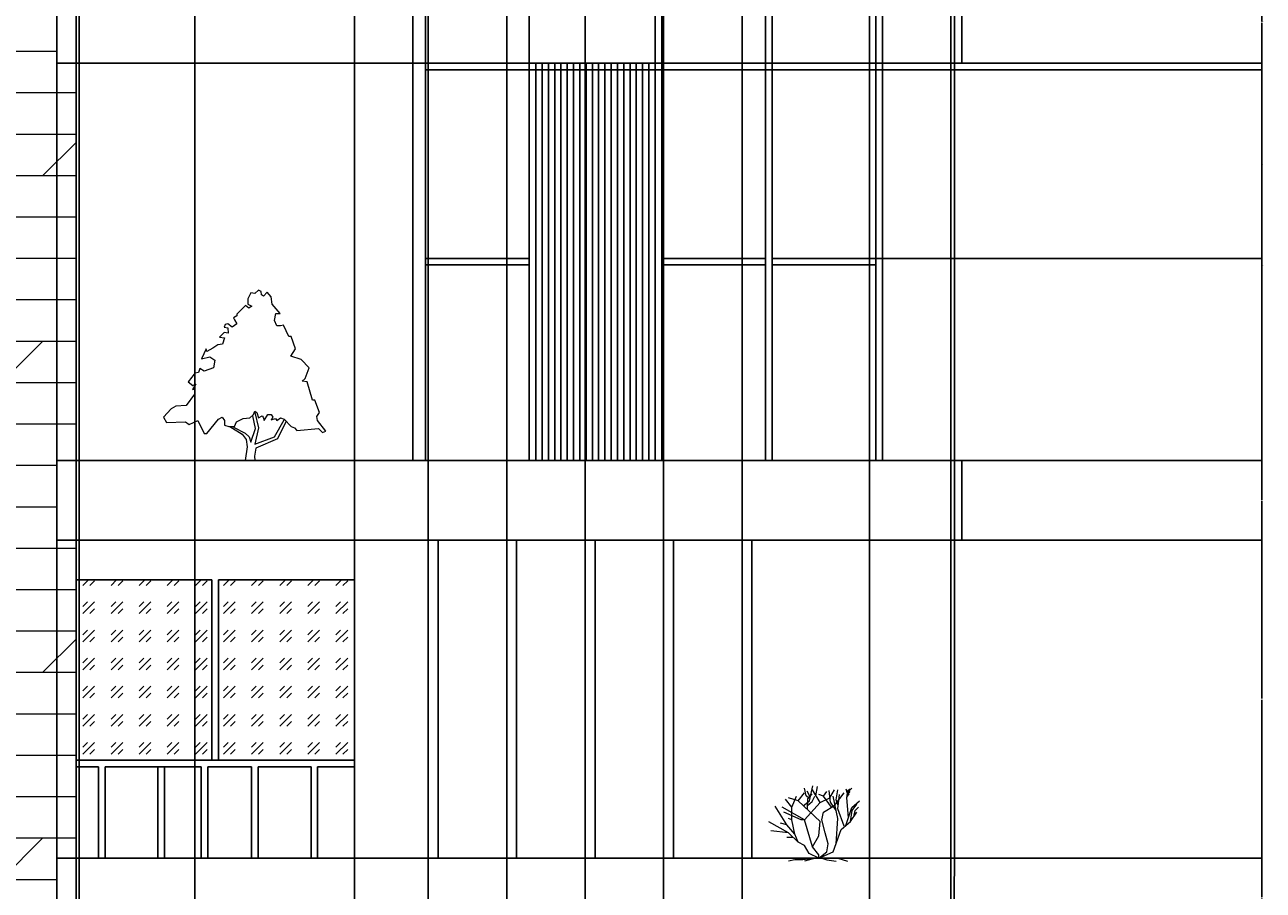
# Model space of a CAD drawing. Units: inches. Extents: x 250 to 1217, y -42 to 832.
# Tile 6 of 7: x 670 to 1043, y 309 to 571. Entities that reach past the tile are written whole.
import ezdxf

# ---------------------------------------------------------------- set-up
doc = ezdxf.new("R2010")
doc.units = ezdxf.units.IN
doc.header["$MEASUREMENT"] = 0
for name, color, linetype, lineweight in [('A-ANNO-DIMS', 2, 'Continuous', 18), ('A-ELEV', 7, 'Continuous', 25), ('A-ELEV-PATT', 8, 'Continuous', 13), ('L-PLNT', 3, 'Continuous', 13)]:
    doc.layers.add(name, color=color, linetype=linetype, lineweight=lineweight)
doc.styles.get("Standard").update_dxf_attribs({"font": 'arial.ttf'})
doc.dimstyles.get("Standard").update_dxf_attribs({"dimtxt": 0.18, "dimasz": 0.18, "dimexe": 0.18, "dimexo": 0.0625, "dimgap": 0.09, "dimtad": 0, "dimtih": 1, "dimtoh": 1, "dimdec": 4, "dimzin": 0, "dimdsep": 46, "dimtxsty": 'Standard', "dimcen": 0.09, "dimadec": 0, "dimazin": 0, "dimtfac": 1, "dimtdec": 4, "dimtofl": 0, "dimtmove": 0, "dimatfit": 3, "dimfxl": 1, "dimtolj": 1, "dimtzin": 0, "dimarcsym": 0})

# ---------------------------------------------------------------- blocks, each defined once
blk = doc.blocks.new('*U2')
for p, q in [((-11.433, 18.289), (-10.457, 22.749)), ((-9.48, 19.775), (-8.992, 22.592)), ((-16.8, 16.32), (-18.72, 18.72)), ((-14.88, 18.24), (-17.76, 19.2)), ((-16.8, 16.32), (-15.36, 19.68)), ((-14.88, 18.24), (-12.96, 20.64)), ((-12.471, 19.775), (-12.898, 22.044)), ((-11.677, 19.071), (-12.471, 19.775)), ((-11.28, 19.619), (-12.104, 21.184)), ((-12.043, 15.628), (-11.921, 18.836)), ((-11.921, 18.836), (-10.64, 20.401)), ((-10.579, 18.054), (-9.846, 19.697)), ((-8.16, 17.76), (-10.56, 21.6)), ((-7.2, 19.68), (-8.64, 20.16)), ((-8.16, 17.76), (-5.28, 19.2)), ((-7.2, 19.68), (-6.24, 21.12)), ((-4.8, 16.32), (-7.2, 19.68)), ((-5.086, 17.741), (-5.513, 21.34)), ((-5.28, 19.2), (-3.84, 21.6)), ((-2.88, 12.96), (-4.32, 19.68)), ((-3.84, 16.8), (-0.96, 20.64)), ((-3.377, 18.602), (-2.888, 21.575)), ((-2.88, 15.84), (-2.4, 20.16)), ((-0.508, 21.888), (-0.081, 20.558)), ((-0.203, 19.149), (0.102, 21.34)), ((0.346, 13.203), (-0.203, 19.149)), ((-0.142, 19.384), (0.59, 20.401)), ((-0.02, 20.01), (0.896, 21.105)), ((0.041, 20.714), (1.384, 22.044)), ((0.102, 21.34), (0.835, 21.888)), ((-18.24, 11.04), (-21.755, 16.655)), ((-12.96, 12.48), (-19.68, 16.32)), ((-16.8, 12.48), (-16.8, 16.32)), ((-8.16, 12), (-14.88, 18.24)), ((-13.325, 16.724), (-11.433, 18.289)), ((-12.96, 12.48), (-8.16, 17.76)), ((-11.982, 16.802), (-10.579, 18.054)), ((-7.2, 14.88), (-3.84, 16.8)), ((-3.377, 15.315), (-5.086, 17.819)), ((-2.766, 16.802), (-3.377, 18.602)), ((-0.96, 10.56), (-2.88, 15.84)), ((0.346, 13.203), (1.323, 16.254)), ((0.96, 12), (1.44, 15.36)), ((1.323, 16.254), (3.642, 18.289)), ((1.44, 15.36), (2.88, 17.28)), ((1.92, 13.44), (2.4, 15.36)), ((2.4, 15.36), (3.36, 16.32)), ((-17.76, 8.64), (-23.663, 11.961)), ((-18.24, 11.04), (-20.16, 11.52)), ((-13.92, 12.48), (-19.2, 14.88)), ((-16.8, 12.48), (-17.76, 12.96)), ((-15.84, 8.16), (-16.8, 12.48)), ((-12.96, 12.48), (-13.92, 12.48)), ((-10.56, 4.32), (-12.96, 12.48)), ((-8.64, 7.68), (-8.16, 12)), ((-7.68, 12.48), (-7.2, 14.88)), ((-6.72, 8.64), (-7.68, 12.48)), ((-3.36, 5.28), (-2.88, 12.96)), ((-1.92, 9.6), (0.96, 12)), ((-0.48, 10.8), (0.346, 13.203)), ((0.96, 12), (2.88, 14.88)), ((-17.76, 8.64), (-23.128, 9.222)), ((-15.84, 8.16), (-18.24, 11.04)), ((-14.88, 5.76), (-17.76, 8.64)), ((-14.88, 5.76), (-15.84, 8.16)), ((-10.56, 4.32), (-8.64, 7.68)), ((-5.76, 5.28), (-6.72, 8.64)), ((-4.32, 2.88), (-1.92, 9.6)), ((-16.32, 7.2), (-18.24, 7.2)), ((-12.96, 4.8), (-14.88, 5.76)), ((-11.52, 2.4), (-12.96, 4.8)), ((-8.64, 1.92), (-10.56, 4.32)), ((-6.24, 2.88), (-5.76, 5.28)), ((-15.84, 0.48), (-17.76, 0)), ((-13.44, 0.48), (-15.84, 0.48)), ((-9.6, 0.96), (-13.44, 0.48)), ((-9.6, 0.96), (-12.96, 0)), ((-8.64, 0.96), (-11.52, 2.4)), ((-9.6, 0.96), (-7.68, 0.96)), ((-8.64, 0.96), (-4.32, 2.88)), ((-8.64, 0.96), (-6.24, 2.88)), ((-8.64, 0.96), (-8.64, 1.92)), ((-8.64, 0.96), (-2.88, 0.96)), ((-7.68, 0.96), (-6.24, 0.48)), ((-6.24, 0.48), (-3.36, 0)), ((-2.88, 0.96), (0, 0))]:
    blk.add_line(p, q)
blk = doc.blocks.new('*U3')
for points in [[(22.0124, 137.721), (18.5475, 141.5624), (15.5282, 138.2446), (13.8028, 139.3505), (13.3714, 142.1153), (11.2148, 143.2214), (8.1954, 140.4564), (4.7447, 141.0094), (2.1567, 136.0326), (2.1567, 131.6088), (5.6074, 129.9499), (3.0193, 128.2909), (0.4313, 130.5029), (-6.9015, 123.3141), (-6.9015, 121.6552), (-9.9208, 119.9963), (-9.0581, 118.3373), (-6.9015, 115.0195), (-10.7835, 112.2546), (-14.6656, 115.0195), (-16.8222, 114.4665), (-17.6849, 112.2546), (-14.6656, 111.7016), (-14.2342, 107.2778), (-17.6065, 107.8307), (-21.5669, 103.9599), (-17.2536, 103.4069), (-18.9789, 97.8771), (-22.8609, 97.3241), (-27.1743, 94.5593), (-32.3504, 91.7944), (-32.7817, 94.0063), (-36.6638, 85.7116), (-29.7624, 87.3705), (-25.449, 84.6056), (-26.743, 77.9699), (-34.507, 75.205), (-37.9578, 77.4169), (-39.2518, 74.099), (-42.2711, 73.5461), (-44.8592, 70.2282), (-47.8786, 66.3574), (-43.9965, 63.0395), (-41.4085, 64.6985), (-44.3346, 59.8898), (-42.2089, 60.1377), (-42.5159, 55.7849), (-49.6039, 46.4502), (-58.2307, 45.8972), (-62.1127, 43.6853), (-68.5828, 36.4966), (-65.9947, 32.0727), (-50.0352, 32.6257), (-47.0159, 30.4138), (-39.6831, 33.7317), (-34.507, 22.6721), (-32.3504, 22.6721), (-22.4296, 34.8376), (-19.4102, 36.4966), (-17.2536, 33.7317), (-17.2536, 29.8608), (-13.8028, 28.7549), (-9.0581, 28.7549), (-7.3328, 32.6257), (-1.7254, 35.3906), (3.8821, 35.9436), (6.4701, 38.1555), (6.9014, 38.7085), (8.1954, 41.4734), (9.9208, 40.3674), (11.2148, 35.9436), (14.2341, 37.6025), (15.0968, 36.4966), (15.9595, 33.7317), (18.9789, 38.7085), (21.9982, 38.7085), (23.2922, 36.4966), (21.9982, 34.2847), (25.4489, 35.3906), (26.743, 33.7317), (29.7623, 35.9436), (32.7817, 34.8376), (38.8204, 28.7549), (41.4084, 27.6489), (43.5651, 25.437), (61.6813, 27.0959), (65.132, 23.7781), (67.7201, 24.884), (60.8186, 33.7317), (60.3873, 37.0495), (62.544, 40.3674), (58.662, 50.874), (56.5053, 50.874), (52.1919, 66.3574), (47.8785, 66.9103), (50.4665, 69.1222), (53.9172, 77.9699), (47.0158, 85.1586), (38.3891, 87.9235), (42.2711, 94.0063)], [(42.2711, 94.0063), (38.8204, 104.5129), (36.6637, 104.5129), (32.3503, 113.9135), (29.7623, 113.3605), (26.743, 113.3605), (24.5862, 117.7844), (25.8802, 123.8671), (29.331, 123.8671), (22.8609, 131.6088), (21.9982, 137.6916)], [(-9.9208, 28.2019), (0, 23.2251), (3.4507, 19.9072), (4.7447, 15.4834), (8.6267, 27.0959), (6.4701, 37.6025)], [(34.5071, 33.1787), (27.1743, 18.2483), (9.0581, 10.5066), (7.7641, 3.8708), (8.1954, 0)], [(8.1954, 40.3674), (11.2148, 27.6489), (8.1954, 13.8245), (24.5862, 19.9072), (32.7817, 34.2847)], [(-12.9401, 28.7549), (-2.588, 22.1191), (0.8626, 17.6953), (1.7253, 11.6125), (0, 0)]]:
    blk.add_lwpolyline(points)
blk = doc.blocks.new('*D15')
at = {"layer": 'A-ANNO-DIMS', "color": 0, "lineweight": -2, "transparency": 16777216}
for p, q in [((950.12, 318.93), (1043.08, 318.93)), ((1042.9, 318.75), (1042.9, 307.11)), ((1042.9, 295.11), (1042.9, 306.75)), ((926.12, 294.93), (1043.08, 294.93))]:
    blk.add_line(p, q, dxfattribs=at)
at = {"layer": 'A-ANNO-DIMS', "color": 0, "transparency": 16777216}
for points in [[(1042.87, 318.75), (1042.93, 318.75), (1042.9, 318.93)], [(1042.87, 295.11), (1042.93, 295.11), (1042.9, 294.93)]]:
    blk.add_solid(points, dxfattribs=at)
at = {"layer": 'Defpoints', "color": 0, "transparency": 16777216}
for p in [(950.06, 318.93), (1042.9, 318.93), (926.06, 294.93)]:
    blk.add_point(p, dxfattribs=at)
at = {"layer": 'A-ANNO-DIMS', "color": 0, "transparency": 16777216, "insert": (1042.9, 306.93), "char_height": 0.18, "attachment_point": 5}
blk.add_mtext('\\A1;24', dxfattribs=at)
blk = doc.blocks.new('*D16')
at = {"layer": 'A-ANNO-DIMS', "color": 0, "lineweight": -2, "transparency": 16777216}
for p, q in [((952.41, 414.93), (1043.08, 414.93)), ((1042.9, 414.75), (1042.9, 367.11)), ((1042.9, 319.11), (1042.9, 366.75)), ((950.12, 318.93), (1043.08, 318.93))]:
    blk.add_line(p, q, dxfattribs=at)
at = {"layer": 'A-ANNO-DIMS', "color": 0, "transparency": 16777216}
for points in [[(1042.87, 414.75), (1042.93, 414.75), (1042.9, 414.93)], [(1042.87, 319.11), (1042.93, 319.11), (1042.9, 318.93)]]:
    blk.add_solid(points, dxfattribs=at)
at = {"layer": 'Defpoints', "color": 0, "transparency": 16777216}
for p in [(952.34, 414.93), (1042.9, 414.93), (950.06, 318.93)]:
    blk.add_point(p, dxfattribs=at)
at = {"layer": 'A-ANNO-DIMS', "color": 0, "transparency": 16777216, "insert": (1042.9, 366.93), "char_height": 0.18, "attachment_point": 5}
blk.add_mtext('\\A1;96', dxfattribs=at)
blk = doc.blocks.new('*D17')
at = {"layer": 'A-ANNO-DIMS', "color": 0, "lineweight": -2, "transparency": 16777216}
for p, q in [((952.41, 438.93), (1043.08, 438.93)), ((1042.9, 438.75), (1042.9, 427.11)), ((1042.9, 415.11), (1042.9, 426.75)), ((952.41, 414.93), (1043.08, 414.93))]:
    blk.add_line(p, q, dxfattribs=at)
at = {"layer": 'A-ANNO-DIMS', "color": 0, "transparency": 16777216}
for points in [[(1042.87, 438.75), (1042.93, 438.75), (1042.9, 438.93)], [(1042.87, 415.11), (1042.93, 415.11), (1042.9, 414.93)]]:
    blk.add_solid(points, dxfattribs=at)
at = {"layer": 'Defpoints', "color": 0, "transparency": 16777216}
for p in [(952.34, 438.93), (1042.9, 438.93), (952.34, 414.93)]:
    blk.add_point(p, dxfattribs=at)
at = {"layer": 'A-ANNO-DIMS', "color": 0, "transparency": 16777216, "insert": (1042.9, 426.93), "char_height": 0.18, "attachment_point": 5}
blk.add_mtext('\\A1;24', dxfattribs=at)
blk = doc.blocks.new('*D18')
at = {"layer": 'A-ANNO-DIMS', "color": 0, "lineweight": -2, "transparency": 16777216}
for p, q in [((952.41, 558.93), (1043.08, 558.93)), ((1042.9, 558.75), (1042.9, 499.11)), ((1042.9, 439.11), (1042.9, 498.75)), ((952.41, 438.93), (1043.08, 438.93))]:
    blk.add_line(p, q, dxfattribs=at)
at = {"layer": 'A-ANNO-DIMS', "color": 0, "transparency": 16777216}
for points in [[(1042.87, 558.75), (1042.93, 558.75), (1042.9, 558.93)], [(1042.87, 439.11), (1042.93, 439.11), (1042.9, 438.93)]]:
    blk.add_solid(points, dxfattribs=at)
at = {"layer": 'Defpoints', "color": 0, "transparency": 16777216}
for p in [(952.34, 558.93), (1042.9, 558.93), (952.34, 438.93)]:
    blk.add_point(p, dxfattribs=at)
at = {"layer": 'A-ANNO-DIMS', "color": 0, "transparency": 16777216, "insert": (1042.9, 498.93), "char_height": 0.18, "attachment_point": 5}
blk.add_mtext('\\A1;120', dxfattribs=at)
blk = doc.blocks.new('*D19')
at = {"layer": 'A-ANNO-DIMS', "color": 0, "lineweight": -2, "transparency": 16777216}
for p, q in [((928.21, 583.67), (1043.08, 583.67)), ((1042.9, 583.49), (1042.9, 571.48)), ((1042.9, 559.11), (1042.9, 571.12)), ((952.41, 558.93), (1043.08, 558.93))]:
    blk.add_line(p, q, dxfattribs=at)
at = {"layer": 'A-ANNO-DIMS', "color": 0, "transparency": 16777216}
for points in [[(1042.87, 583.49), (1042.93, 583.49), (1042.9, 583.67)], [(1042.87, 559.11), (1042.93, 559.11), (1042.9, 558.93)]]:
    blk.add_solid(points, dxfattribs=at)
at = {"layer": 'Defpoints', "color": 0, "transparency": 16777216}
for p in [(928.15, 583.67), (1042.9, 583.67), (952.34, 558.93)]:
    blk.add_point(p, dxfattribs=at)
at = {"layer": 'A-ANNO-DIMS', "color": 0, "transparency": 16777216, "insert": (1042.9, 571.3), "char_height": 0.18, "attachment_point": 5}
blk.add_mtext('\\A1;24.747', dxfattribs=at)
blk = doc.blocks.new('*D27')
at = {"layer": 'A-ANNO-DIMS', "color": 0, "lineweight": -2, "transparency": 16777216}
for p, q in [((624.98, 174.99), (624.98, 831.77)), ((625.16, 831.59), (655.07, 831.59)), ((685.76, 831.59), (655.86, 831.59)), ((685.94, 176.49), (685.94, 831.77))]:
    blk.add_line(p, q, dxfattribs=at)
at = {"layer": 'A-ANNO-DIMS', "color": 0, "transparency": 16777216}
for points in [[(625.16, 831.62), (625.16, 831.56), (624.98, 831.59)], [(685.76, 831.62), (685.76, 831.56), (685.94, 831.59)]]:
    blk.add_solid(points, dxfattribs=at)
at = {"layer": 'Defpoints', "color": 0, "transparency": 16777216}
for p in [(685.94, 831.59), (685.94, 176.43), (624.98, 174.93)]:
    blk.add_point(p, dxfattribs=at)
at = {"layer": 'A-ANNO-DIMS', "color": 0, "transparency": 16777216, "insert": (655.46, 831.59), "char_height": 0.18, "attachment_point": 5}
blk.add_mtext('\\A1;60.96', dxfattribs=at)
blk = doc.blocks.new('*D28')
at = {"layer": 'A-ANNO-DIMS', "color": 0, "lineweight": -2, "transparency": 16777216}
for p, q in [((685.94, 176.49), (685.94, 831.77)), ((686.12, 831.59), (727.07, 831.59)), ((768.8, 831.59), (727.86, 831.59)), ((768.98, 162.99), (768.98, 831.77))]:
    blk.add_line(p, q, dxfattribs=at)
at = {"layer": 'A-ANNO-DIMS', "color": 0, "transparency": 16777216}
for points in [[(686.12, 831.62), (686.12, 831.56), (685.94, 831.59)], [(768.8, 831.62), (768.8, 831.56), (768.98, 831.59)]]:
    blk.add_solid(points, dxfattribs=at)
at = {"layer": 'Defpoints', "color": 0, "transparency": 16777216}
for p in [(768.98, 831.59), (685.94, 176.43), (768.98, 162.93)]:
    blk.add_point(p, dxfattribs=at)
at = {"layer": 'A-ANNO-DIMS', "color": 0, "transparency": 16777216, "insert": (727.46, 831.59), "char_height": 0.18, "attachment_point": 5}
blk.add_mtext('\\A1;83.04', dxfattribs=at)
blk = doc.blocks.new('*D29')
at = {"layer": 'A-ANNO-DIMS', "color": 0, "lineweight": -2, "transparency": 16777216}
for p, q in [((768.98, 162.99), (768.98, 831.77)), ((769.16, 831.59), (779.67, 831.59)), ((791.11, 831.59), (780.6, 831.59)), ((791.29, 174.99), (791.29, 831.77))]:
    blk.add_line(p, q, dxfattribs=at)
at = {"layer": 'A-ANNO-DIMS', "color": 0, "transparency": 16777216}
for points in [[(769.16, 831.62), (769.16, 831.56), (768.98, 831.59)], [(791.11, 831.62), (791.11, 831.56), (791.29, 831.59)]]:
    blk.add_solid(points, dxfattribs=at)
at = {"layer": 'Defpoints', "color": 0, "transparency": 16777216}
for p in [(791.29, 831.59), (791.29, 174.93), (768.98, 162.93)]:
    blk.add_point(p, dxfattribs=at)
at = {"layer": 'A-ANNO-DIMS', "color": 0, "transparency": 16777216, "insert": (780.13, 831.59), "char_height": 0.18, "attachment_point": 5}
blk.add_mtext('\\A1;22.303', dxfattribs=at)
blk = doc.blocks.new('*D30')
at = {"layer": 'A-ANNO-DIMS', "color": 0, "lineweight": -2, "transparency": 16777216}
for p, q in [((814.96, 174.99), (814.96, 831.77)), ((815.14, 831.59), (826.33, 831.59)), ((838.45, 831.59), (827.26, 831.59)), ((838.63, 174.99), (838.63, 831.77))]:
    blk.add_line(p, q, dxfattribs=at)
at = {"layer": 'A-ANNO-DIMS', "color": 0, "transparency": 16777216}
for points in [[(815.14, 831.62), (815.14, 831.56), (814.96, 831.59)], [(838.45, 831.62), (838.45, 831.56), (838.63, 831.59)]]:
    blk.add_solid(points, dxfattribs=at)
at = {"layer": 'Defpoints', "color": 0, "transparency": 16777216}
for p in [(838.63, 831.59), (814.96, 174.93), (838.63, 174.93)]:
    blk.add_point(p, dxfattribs=at)
at = {"layer": 'A-ANNO-DIMS', "color": 0, "transparency": 16777216, "insert": (826.8, 831.59), "char_height": 0.18, "attachment_point": 5}
blk.add_mtext('\\A1;23.674', dxfattribs=at)
blk = doc.blocks.new('*D31')
at = {"layer": 'A-ANNO-DIMS', "color": 0, "lineweight": -2, "transparency": 16777216}
for p, q in [((862.31, 174.99), (862.31, 831.77)), ((862.49, 831.59), (873.68, 831.59)), ((885.8, 831.59), (874.61, 831.59)), ((885.98, 174.99), (885.98, 831.77))]:
    blk.add_line(p, q, dxfattribs=at)
at = {"layer": 'A-ANNO-DIMS', "color": 0, "transparency": 16777216}
for points in [[(862.49, 831.62), (862.49, 831.56), (862.31, 831.59)], [(885.8, 831.62), (885.8, 831.56), (885.98, 831.59)]]:
    blk.add_solid(points, dxfattribs=at)
at = {"layer": 'Defpoints', "color": 0, "transparency": 16777216}
for p in [(885.98, 831.59), (862.31, 174.93), (885.98, 174.93)]:
    blk.add_point(p, dxfattribs=at)
at = {"layer": 'A-ANNO-DIMS', "color": 0, "transparency": 16777216, "insert": (874.15, 831.59), "char_height": 0.18, "attachment_point": 5}
blk.add_mtext('\\A1;23.674', dxfattribs=at)
blk = doc.blocks.new('*D32')
at = {"layer": 'A-ANNO-DIMS', "color": 0, "lineweight": -2, "transparency": 16777216}
for p, q in [((885.98, 174.99), (885.98, 831.77)), ((886.16, 831.59), (917.26, 831.59)), ((948.8, 831.59), (917.7, 831.59)), ((948.98, 174.99), (948.98, 831.77))]:
    blk.add_line(p, q, dxfattribs=at)
at = {"layer": 'A-ANNO-DIMS', "color": 0, "transparency": 16777216}
for points in [[(886.16, 831.62), (886.16, 831.56), (885.98, 831.59)], [(948.8, 831.62), (948.8, 831.56), (948.98, 831.59)]]:
    blk.add_solid(points, dxfattribs=at)
at = {"layer": 'Defpoints', "color": 0, "transparency": 16777216}
for p in [(948.98, 831.59), (885.98, 174.93), (948.98, 174.93)]:
    blk.add_point(p, dxfattribs=at)
at = {"layer": 'A-ANNO-DIMS', "color": 0, "transparency": 16777216, "insert": (917.48, 831.59), "char_height": 0.18, "attachment_point": 5}
blk.add_mtext('\\A1;63', dxfattribs=at)
blk = doc.blocks.new('*D33')
at = {"layer": 'A-ANNO-DIMS', "color": 0, "lineweight": -2, "transparency": 16777216}
for p, q in [((791.29, 414.99), (791.29, 831.77)), ((791.47, 831.59), (802.66, 831.59)), ((814.78, 831.59), (803.59, 831.59)), ((814.96, 414.99), (814.96, 831.77))]:
    blk.add_line(p, q, dxfattribs=at)
at = {"layer": 'A-ANNO-DIMS', "color": 0, "transparency": 16777216}
for points in [[(791.47, 831.62), (791.47, 831.56), (791.29, 831.59)], [(814.78, 831.62), (814.78, 831.56), (814.96, 831.59)]]:
    blk.add_solid(points, dxfattribs=at)
at = {"layer": 'Defpoints', "color": 0, "transparency": 16777216}
for p in [(814.96, 831.59), (791.29, 414.93), (814.96, 414.93)]:
    blk.add_point(p, dxfattribs=at)
at = {"layer": 'A-ANNO-DIMS', "color": 0, "transparency": 16777216, "insert": (803.12, 831.59), "char_height": 0.18, "attachment_point": 5}
blk.add_mtext('\\A1;23.674', dxfattribs=at)
blk = doc.blocks.new('*D34')
at = {"layer": 'A-ANNO-DIMS', "color": 0, "lineweight": -2, "transparency": 16777216}
for p, q in [((838.63, 414.99), (838.63, 831.77)), ((838.81, 831.59), (850.01, 831.59)), ((862.13, 831.59), (850.94, 831.59)), ((862.31, 414.99), (862.31, 831.77))]:
    blk.add_line(p, q, dxfattribs=at)
at = {"layer": 'A-ANNO-DIMS', "color": 0, "transparency": 16777216}
for points in [[(838.81, 831.62), (838.81, 831.56), (838.63, 831.59)], [(862.13, 831.62), (862.13, 831.56), (862.31, 831.59)]]:
    blk.add_solid(points, dxfattribs=at)
at = {"layer": 'Defpoints', "color": 0, "transparency": 16777216}
for p in [(862.31, 831.59), (838.63, 414.93), (862.31, 414.93)]:
    blk.add_point(p, dxfattribs=at)
at = {"layer": 'A-ANNO-DIMS', "color": 0, "transparency": 16777216, "insert": (850.47, 831.59), "char_height": 0.18, "attachment_point": 5}
blk.add_mtext('\\A1;23.674', dxfattribs=at)
blk = doc.blocks.new('*D37')
at = {"layer": 'A-ANNO-DIMS', "color": 0, "lineweight": -2, "transparency": 16777216}
for p, q in [((926.42, 499.99), (1043.08, 499.99)), ((1042.9, 499.81), (1042.9, 469.64)), ((1042.9, 439.11), (1042.9, 469.28)), ((928.42, 438.93), (1043.08, 438.93))]:
    blk.add_line(p, q, dxfattribs=at)
at = {"layer": 'A-ANNO-DIMS', "color": 0, "transparency": 16777216}
for points in [[(1042.87, 499.81), (1042.93, 499.81), (1042.9, 499.99)], [(1042.87, 439.11), (1042.93, 439.11), (1042.9, 438.93)]]:
    blk.add_solid(points, dxfattribs=at)
at = {"layer": 'Defpoints', "color": 0, "transparency": 16777216}
for p in [(926.36, 499.99), (1042.9, 499.99), (928.36, 438.93)]:
    blk.add_point(p, dxfattribs=at)
at = {"layer": 'A-ANNO-DIMS', "color": 0, "transparency": 16777216, "insert": (1042.9, 469.46), "char_height": 0.18, "attachment_point": 5}
blk.add_mtext('\\A1;61.06', dxfattribs=at)
blk = doc.blocks.new('*D50')
at = {"layer": 'A-ANNO-DIMS', "color": 0, "lineweight": -2, "transparency": 16777216}
for p, q in [((679.19, 318.99), (679.19, 831.77)), ((679.37, 831.59), (814.16, 831.59)), ((949.88, 831.59), (815.09, 831.59)), ((950.06, 318.99), (950.06, 831.77))]:
    blk.add_line(p, q, dxfattribs=at)
at = {"layer": 'A-ANNO-DIMS', "color": 0, "transparency": 16777216}
for points in [[(679.37, 831.62), (679.37, 831.56), (679.19, 831.59)], [(949.88, 831.62), (949.88, 831.56), (950.06, 831.59)]]:
    blk.add_solid(points, dxfattribs=at)
at = {"layer": 'Defpoints', "color": 0, "transparency": 16777216}
for p in [(950.06, 831.59), (679.19, 318.93), (950.06, 318.93)]:
    blk.add_point(p, dxfattribs=at)
at = {"layer": 'A-ANNO-DIMS', "color": 0, "transparency": 16777216, "insert": (814.62, 831.59), "char_height": 0.18, "attachment_point": 5}
blk.add_mtext('\\A1;270.87', dxfattribs=at)
blk = doc.blocks.new('*D52')
at = {"layer": 'A-ANNO-DIMS', "color": 0, "lineweight": -2, "transparency": 16777216}
for p, q in [((924.49, 199.65), (924.49, 831.77)), ((924.67, 831.59), (936.34, 831.59)), ((948.8, 831.59), (937.13, 831.59)), ((948.98, 198.99), (948.98, 831.77))]:
    blk.add_line(p, q, dxfattribs=at)
at = {"layer": 'A-ANNO-DIMS', "color": 0, "transparency": 16777216}
for points in [[(924.67, 831.62), (924.67, 831.56), (924.49, 831.59)], [(948.8, 831.62), (948.8, 831.56), (948.98, 831.59)]]:
    blk.add_solid(points, dxfattribs=at)
at = {"layer": 'Defpoints', "color": 0, "transparency": 16777216}
for p in [(948.98, 831.59), (924.49, 199.59), (948.98, 198.93)]:
    blk.add_point(p, dxfattribs=at)
at = {"layer": 'A-ANNO-DIMS', "color": 0, "transparency": 16777216, "insert": (936.74, 831.59), "char_height": 0.18, "attachment_point": 5}
blk.add_mtext('\\A1;24.49', dxfattribs=at)
blk = doc.blocks.new('*D55')
at = {"layer": 'A-ANNO-DIMS', "color": 0, "lineweight": -2, "transparency": 16777216}
for p, q in [((684.98, 438.99), (684.98, 831.77)), ((685.16, 831.59), (735.35, 831.59)), ((786.44, 831.59), (736.26, 831.59)), ((786.62, 438.99), (786.62, 831.77))]:
    blk.add_line(p, q, dxfattribs=at)
at = {"layer": 'A-ANNO-DIMS', "color": 0, "transparency": 16777216}
for points in [[(685.16, 831.62), (685.16, 831.56), (684.98, 831.59)], [(786.44, 831.62), (786.44, 831.56), (786.62, 831.59)]]:
    blk.add_solid(points, dxfattribs=at)
at = {"layer": 'Defpoints', "color": 0, "transparency": 16777216}
for p in [(786.62, 831.59), (684.98, 438.93), (786.62, 438.93)]:
    blk.add_point(p, dxfattribs=at)
at = {"layer": 'A-ANNO-DIMS', "color": 0, "transparency": 16777216, "insert": (735.8, 831.59), "char_height": 0.18, "attachment_point": 5}
blk.add_mtext('\\A1;101.64', dxfattribs=at)
blk = doc.blocks.new('*D56')
at = {"layer": 'A-ANNO-DIMS', "color": 0, "lineweight": -2, "transparency": 16777216}
for p, q in [((786.62, 438.99), (786.62, 831.77)), ((786.8, 831.59), (803.8, 831.59)), ((821.58, 831.59), (804.59, 831.59)), ((821.76, 438.99), (821.76, 831.77))]:
    blk.add_line(p, q, dxfattribs=at)
at = {"layer": 'A-ANNO-DIMS', "color": 0, "transparency": 16777216}
for points in [[(786.8, 831.62), (786.8, 831.56), (786.62, 831.59)], [(821.58, 831.62), (821.58, 831.56), (821.76, 831.59)]]:
    blk.add_solid(points, dxfattribs=at)
at = {"layer": 'Defpoints', "color": 0, "transparency": 16777216}
for p in [(821.76, 831.59), (786.62, 438.93), (821.76, 438.93)]:
    blk.add_point(p, dxfattribs=at)
at = {"layer": 'A-ANNO-DIMS', "color": 0, "transparency": 16777216, "insert": (804.19, 831.59), "char_height": 0.18, "attachment_point": 5}
blk.add_mtext('\\A1;35.14', dxfattribs=at)
blk = doc.blocks.new('*D57')
at = {"layer": 'A-ANNO-DIMS', "color": 0, "lineweight": -2, "transparency": 16777216}
for p, q in [((821.76, 438.99), (821.76, 831.77)), ((821.94, 831.59), (840.54, 831.59)), ((859.58, 831.59), (840.98, 831.59)), ((859.76, 438.99), (859.76, 831.77))]:
    blk.add_line(p, q, dxfattribs=at)
at = {"layer": 'A-ANNO-DIMS', "color": 0, "transparency": 16777216}
for points in [[(821.94, 831.62), (821.94, 831.56), (821.76, 831.59)], [(859.58, 831.62), (859.58, 831.56), (859.76, 831.59)]]:
    blk.add_solid(points, dxfattribs=at)
at = {"layer": 'Defpoints', "color": 0, "transparency": 16777216}
for p in [(859.76, 831.59), (821.76, 438.93), (859.76, 438.93)]:
    blk.add_point(p, dxfattribs=at)
at = {"layer": 'A-ANNO-DIMS', "color": 0, "transparency": 16777216, "insert": (840.76, 831.59), "char_height": 0.18, "attachment_point": 5}
blk.add_mtext('\\A1;38', dxfattribs=at)
blk = doc.blocks.new('*D58')
at = {"layer": 'A-ANNO-DIMS', "color": 0, "lineweight": -2, "transparency": 16777216}
for p, q in [((859.76, 438.99), (859.76, 831.77)), ((859.94, 831.59), (893.74, 831.59)), ((928.18, 831.59), (894.39, 831.59)), ((928.36, 438.99), (928.36, 831.77))]:
    blk.add_line(p, q, dxfattribs=at)
at = {"layer": 'A-ANNO-DIMS', "color": 0, "transparency": 16777216}
for points in [[(859.94, 831.62), (859.94, 831.56), (859.76, 831.59)], [(928.18, 831.62), (928.18, 831.56), (928.36, 831.59)]]:
    blk.add_solid(points, dxfattribs=at)
at = {"layer": 'Defpoints', "color": 0, "transparency": 16777216}
for p in [(928.36, 831.59), (859.76, 438.93), (928.36, 438.93)]:
    blk.add_point(p, dxfattribs=at)
at = {"layer": 'A-ANNO-DIMS', "color": 0, "transparency": 16777216, "insert": (894.06, 831.59), "char_height": 0.18, "attachment_point": 5}
blk.add_mtext('\\A1;68.6', dxfattribs=at)
blk = doc.blocks.new('*D87')
at = {"layer": 'A-ANNO-DIMS', "color": 0, "lineweight": -2, "transparency": 16777216}
for p, q in [((790.46, 438.99), (790.46, 831.77)), ((790.64, 831.59), (805.72, 831.59)), ((821.58, 831.59), (806.51, 831.59)), ((821.76, 438.99), (821.76, 831.77))]:
    blk.add_line(p, q, dxfattribs=at)
at = {"layer": 'A-ANNO-DIMS', "color": 0, "transparency": 16777216}
for points in [[(790.64, 831.62), (790.64, 831.56), (790.46, 831.59)], [(821.58, 831.62), (821.58, 831.56), (821.76, 831.59)]]:
    blk.add_solid(points, dxfattribs=at)
at = {"layer": 'Defpoints', "color": 0, "transparency": 16777216}
for p in [(821.76, 831.59), (790.46, 438.93), (821.76, 438.93)]:
    blk.add_point(p, dxfattribs=at)
at = {"layer": 'A-ANNO-DIMS', "color": 0, "transparency": 16777216, "insert": (806.11, 831.59), "char_height": 0.18, "attachment_point": 5}
blk.add_mtext('\\A1;31.30', dxfattribs=at)
blk = doc.blocks.new('*D88')
at = {"layer": 'A-ANNO-DIMS', "color": 0, "lineweight": -2, "transparency": 16777216}
for p, q in [((861.76, 438.99), (861.76, 831.77)), ((861.94, 831.59), (877.02, 831.59)), ((892.88, 831.59), (877.81, 831.59)), ((893.06, 438.99), (893.06, 831.77))]:
    blk.add_line(p, q, dxfattribs=at)
at = {"layer": 'A-ANNO-DIMS', "color": 0, "transparency": 16777216}
for points in [[(861.94, 831.62), (861.94, 831.56), (861.76, 831.59)], [(892.88, 831.62), (892.88, 831.56), (893.06, 831.59)]]:
    blk.add_solid(points, dxfattribs=at)
at = {"layer": 'Defpoints', "color": 0, "transparency": 16777216}
for p in [(893.06, 831.59), (861.76, 438.93), (893.06, 438.93)]:
    blk.add_point(p, dxfattribs=at)
at = {"layer": 'A-ANNO-DIMS', "color": 0, "transparency": 16777216, "insert": (877.41, 831.59), "char_height": 0.18, "attachment_point": 5}
blk.add_mtext('\\A1;31.30', dxfattribs=at)
blk = doc.blocks.new('*D89')
at = {"layer": 'A-ANNO-DIMS', "color": 0, "lineweight": -2, "transparency": 16777216}
for p, q in [((893.06, 438.99), (893.06, 831.77)), ((893.24, 831.59), (893.74, 831.59)), ((894.88, 831.59), (894.39, 831.59)), ((895.06, 438.99), (895.06, 831.77))]:
    blk.add_line(p, q, dxfattribs=at)
at = {"layer": 'A-ANNO-DIMS', "color": 0, "transparency": 16777216}
for points in [[(893.24, 831.62), (893.24, 831.56), (893.06, 831.59)], [(894.88, 831.62), (894.88, 831.56), (895.06, 831.59)]]:
    blk.add_solid(points, dxfattribs=at)
at = {"layer": 'Defpoints', "color": 0, "transparency": 16777216}
for p in [(895.06, 831.59), (893.06, 438.93), (895.06, 438.93)]:
    blk.add_point(p, dxfattribs=at)
at = {"layer": 'A-ANNO-DIMS', "color": 0, "transparency": 16777216, "insert": (894.06, 831.59), "char_height": 0.18, "attachment_point": 5}
blk.add_mtext('\\A1;2.00', dxfattribs=at)
blk = doc.blocks.new('*D90')
at = {"layer": 'A-ANNO-DIMS', "color": 0, "lineweight": -2, "transparency": 16777216}
for p, q in [((895.06, 438.99), (895.06, 831.77)), ((895.24, 831.59), (910.32, 831.59)), ((926.18, 831.59), (911.11, 831.59)), ((926.36, 438.99), (926.36, 831.77))]:
    blk.add_line(p, q, dxfattribs=at)
at = {"layer": 'A-ANNO-DIMS', "color": 0, "transparency": 16777216}
for points in [[(895.24, 831.62), (895.24, 831.56), (895.06, 831.59)], [(926.18, 831.62), (926.18, 831.56), (926.36, 831.59)]]:
    blk.add_solid(points, dxfattribs=at)
at = {"layer": 'Defpoints', "color": 0, "transparency": 16777216}
for p in [(926.36, 831.59), (895.06, 438.93), (926.36, 438.93)]:
    blk.add_point(p, dxfattribs=at)
at = {"layer": 'A-ANNO-DIMS', "color": 0, "transparency": 16777216, "insert": (910.71, 831.59), "char_height": 0.18, "attachment_point": 5}
blk.add_mtext('\\A1;31.30', dxfattribs=at)
blk = doc.blocks.new('*D91')
at = {"layer": 'A-ANNO-DIMS', "color": 0, "lineweight": -2, "transparency": 16777216}
for p, q in [((926.42, 556.93), (1043.08, 556.93)), ((1042.9, 556.75), (1042.9, 528.64)), ((1042.9, 500.17), (1042.9, 528.28)), ((926.42, 499.99), (1043.08, 499.99))]:
    blk.add_line(p, q, dxfattribs=at)
at = {"layer": 'A-ANNO-DIMS', "color": 0, "transparency": 16777216}
for points in [[(1042.87, 556.75), (1042.93, 556.75), (1042.9, 556.93)], [(1042.87, 500.17), (1042.93, 500.17), (1042.9, 499.99)]]:
    blk.add_solid(points, dxfattribs=at)
at = {"layer": 'Defpoints', "color": 0, "transparency": 16777216}
for p in [(926.36, 556.93), (1042.9, 556.93), (926.36, 499.99)]:
    blk.add_point(p, dxfattribs=at)
at = {"layer": 'A-ANNO-DIMS', "color": 0, "transparency": 16777216, "insert": (1042.9, 528.46), "char_height": 0.18, "attachment_point": 5}
blk.add_mtext('\\A1;56.94', dxfattribs=at)
blk = doc.blocks.new('*D92')
at = {"layer": 'A-ANNO-DIMS', "color": 0, "lineweight": -2, "transparency": 16777216}
for p, q in [((790.53, 556.93), (1043.08, 556.93)), ((1042.9, 556.75), (1042.9, 498.11)), ((1042.9, 439.11), (1042.9, 497.75)), ((790.53, 438.93), (1043.08, 438.93))]:
    blk.add_line(p, q, dxfattribs=at)
at = {"layer": 'A-ANNO-DIMS', "color": 0, "transparency": 16777216}
for points in [[(1042.87, 556.75), (1042.93, 556.75), (1042.9, 556.93)], [(1042.87, 439.11), (1042.93, 439.11), (1042.9, 438.93)]]:
    blk.add_solid(points, dxfattribs=at)
at = {"layer": 'Defpoints', "color": 0, "transparency": 16777216}
for p in [(790.46, 556.93), (1042.9, 556.93), (790.46, 438.93)]:
    blk.add_point(p, dxfattribs=at)
at = {"layer": 'A-ANNO-DIMS', "color": 0, "transparency": 16777216, "insert": (1042.9, 497.93), "char_height": 0.18, "attachment_point": 5}
blk.add_mtext('\\A1;118.00', dxfattribs=at)
blk = doc.blocks.new('*D98')
at = {"layer": 'A-ANNO-DIMS', "color": 0, "lineweight": -2, "transparency": 16777216}
for p, q in [((720.87, 583.82), (720.87, -41.6)), ((685.06, 582.86), (685.06, -41.6)), ((685.24, -41.42), (702.59, -41.42)), ((720.69, -41.42), (703.34, -41.42))]:
    blk.add_line(p, q, dxfattribs=at)
at = {"layer": 'A-ANNO-DIMS', "color": 0, "transparency": 16777216}
for points in [[(685.24, -41.39), (685.24, -41.45), (685.06, -41.42)], [(720.69, -41.39), (720.69, -41.45), (720.87, -41.42)]]:
    blk.add_solid(points, dxfattribs=at)
at = {"layer": 'Defpoints', "color": 0, "transparency": 16777216}
for p in [(720.87, 583.89), (685.06, 582.93), (720.87, -41.42)]:
    blk.add_point(p, dxfattribs=at)
at = {"layer": 'A-ANNO-DIMS', "color": 0, "transparency": 16777216, "insert": (702.97, -41.42), "char_height": 0.18, "attachment_point": 5}
blk.add_mtext('\\A1;35.81', dxfattribs=at)

msp = doc.modelspace()

# ---------------------------------------------------------------- hatches: boundary and pattern name
at = {"layer": 'A-ELEV-PATT'}
h = msp.add_hatch(dxfattribs=at)
h.set_pattern_fill('DOLMIT', color=256, scale=50)
h.paths.add_polyline_path([(684.9826, 558.9271), (679.1872, 558.9271), (679.1872, 582.9271), (685.0649, 582.9271), (685.0649, 678.9271), (679.1872, 678.9271), (679.1872, 702.9271), (630.7779, 702.9271), (630.7779, 678.9271), (625.0649, 678.9271), (625.0649, 582.9271), (630.7779, 582.9271), (630.7779, 558.9271), (624.9826, 558.9271), (624.9826, 438.9271), (630.7779, 438.9271), (630.7779, 414.9271), (624.9826, 414.9271), (624.9826, 318.9271), (630.7779, 318.9271), (630.7779, 294.9271), (624.9826, 294.9271), (624.9826, 198.9271), (630.7779, 198.9271), (630.7779, 174.9271), (624.9826, 174.9271), (624.9826, 78.9271), (684.9826, 78.9271), (684.9826, 174.9271), (679.1872, 174.9271), (679.1872, 198.9271), (683.6004, 198.9271), (684.9826, 198.9271), (684.9826, 294.9271), (679.1872, 294.9271), (679.1872, 318.9271), (684.9826, 318.9271), (684.9826, 414.9271), (679.1872, 414.9271), (679.1872, 438.9271), (684.9826, 438.9271)])
h = msp.add_hatch(dxfattribs=at)
h.set_pattern_fill('GOST_GLASS', color=256)
h.set_pattern_definition([(45, (144, 240), (8.48528, 0), [5, -7]), (45, (146.1213, 240), (8.48528, 0), [2, -10]), (45, (144, 242.1213), (8.48528, 0), [2, -10])])
h.paths.add_polyline_path([(725.9826, 402.9271), (684.9826, 402.9271), (684.9826, 348.4651), (722.7563, 348.4651), (725.9826, 348.4651)])
h.paths.add_polyline_path([(768.9826, 402.9271), (727.9826, 402.9271), (727.9826, 348.4651), (768.9826, 348.4651)])

# ---------------------------------------------------------------- linework, layer by layer
at = {"layer": 'A-ELEV'}
for p, q in [((679.1872, 582.9271), (679.1872, 558.9271)), ((952.3429, 558.9271), (952.3429, 582.9271)), ((679.1872, 558.9271), (952.3429, 558.9271)), ((684.9826, 558.9271), (684.9826, 438.9271)), ((786.6216, 438.9271), (786.6216, 558.9271)), ((790.4641, 499.991), (790.4641, 556.9271)), ((821.7635, 499.991), (821.7635, 556.9271)), ((823.7635, 558.9271), (823.7635, 438.9271)), ((825.6582, 558.9271), (825.6582, 438.9271)), ((827.5529, 558.9271), (827.5529, 438.9271)), ((829.4477, 558.9271), (829.4477, 438.9271)), ((831.3424, 558.9271), (831.3424, 438.9271)), ((833.2371, 558.9271), (833.2371, 438.9271)), ((835.1319, 558.9271), (835.1319, 438.9271)), ((837.0266, 558.9271), (837.0266, 438.9271)), ((838.9213, 558.9271), (838.9213, 438.9271)), ((840.8161, 558.9271), (840.8161, 438.9271)), ((842.7108, 558.9271), (842.7108, 438.9271)), ((844.6056, 558.9271), (844.6056, 438.9271)), ((846.5003, 558.9271), (846.5003, 438.9271)), ((848.395, 558.9271), (848.395, 438.9271)), ((850.2898, 558.9271), (850.2898, 438.9271)), ((852.1845, 558.9271), (852.1845, 438.9271)), ((854.0792, 558.9271), (854.0792, 438.9271)), ((855.974, 558.9271), (855.974, 438.9271)), ((857.8687, 558.9271), (857.8687, 438.9271)), ((859.7635, 558.9271), (859.7635, 438.9271)), ((859.7635, 558.9271), (859.7635, 438.9271)), ((859.7635, 558.9271), (859.7635, 438.9271)), ((859.7635, 558.9271), (859.7635, 438.9271)), ((861.7635, 499.991), (861.7635, 556.9271)), ((893.0628, 499.991), (893.0628, 556.9271)), ((895.0628, 499.991), (895.0628, 556.9271)), ((926.3621, 499.991), (926.3621, 556.9271)), ((928.3621, 438.9271), (928.3621, 558.9271)), ((790.4641, 499.991), (821.7635, 499.991)), ((790.4641, 438.9271), (790.4641, 497.991)), ((790.4641, 497.991), (821.7635, 497.991)), ((821.7635, 438.9271), (821.7635, 497.991)), ((861.7635, 499.991), (893.0628, 499.991)), ((861.7635, 438.9271), (861.7635, 497.991)), ((861.7635, 497.991), (893.0628, 497.991)), ((893.0628, 438.9271), (893.0628, 497.991)), ((895.0628, 499.991), (926.3621, 499.991)), ((895.0628, 438.9271), (895.0628, 497.991)), ((895.0628, 497.991), (926.3621, 497.991)), ((926.3621, 438.9271), (926.3621, 497.991)), ((679.1872, 438.9271), (679.1872, 414.9271)), ((679.1872, 438.9271), (952.3429, 438.9271)), ((952.3429, 438.9271), (952.3429, 414.9271)), ((679.1872, 414.9271), (952.3429, 414.9271)), ((679.1872, 414.9271), (888.9826, 414.9271)), ((684.9826, 414.9271), (684.9826, 318.9271)), ((791.2851, 414.9271), (791.2851, 318.9271)), ((794.2851, 414.9271), (794.2851, 318.9271)), ((814.9595, 414.9271), (814.9595, 318.9271)), ((817.9595, 414.9271), (817.9595, 318.9271)), ((838.6339, 414.9271), (838.6339, 318.9271)), ((841.6339, 414.9271), (841.6339, 318.9271)), ((862.3082, 414.9271), (862.3082, 318.9271)), ((865.3082, 414.9271), (865.3082, 318.9271)), ((885.9826, 414.9271), (885.9826, 318.9271)), ((888.9826, 414.9271), (888.9826, 318.9271)), ((725.9826, 402.9271), (684.9826, 402.9271)), ((725.9826, 402.9271), (725.9826, 348.4651)), ((727.9826, 402.9271), (727.9826, 348.4651)), ((727.9826, 402.9271), (768.9826, 402.9271)), ((768.9826, 402.9271), (727.9826, 402.9271)), ((768.9826, 402.9271), (768.9826, 318.9271)), ((722.7563, 348.4651), (684.9826, 348.4651)), ((768.9826, 348.4651), (708.9826, 348.4651)), ((691.7563, 346.4651), (684.9826, 346.4651)), ((691.7563, 346.4651), (691.7563, 318.9271)), ((693.7563, 346.4651), (693.7563, 318.9271)), ((709.684, 346.4651), (693.7563, 346.4651)), ((722.7563, 346.4651), (708.9826, 346.4651)), ((709.684, 346.4651), (709.684, 318.9271)), ((722.7563, 346.4651), (711.684, 346.4651)), ((711.684, 346.4651), (711.684, 318.9271)), ((722.7563, 346.4651), (722.7563, 318.9271)), ((737.9826, 346.4651), (724.7563, 346.4651)), ((724.7563, 346.4651), (724.7563, 318.9271)), ((737.9826, 346.4651), (737.9826, 318.9271)), ((739.9826, 346.4651), (739.9826, 318.9271)), ((755.9103, 346.4651), (739.9826, 346.4651)), ((755.9103, 346.4651), (755.9103, 318.9271)), ((768.9826, 346.4651), (757.9103, 346.4651)), ((757.9103, 346.4651), (757.9103, 318.9271)), ((679.1872, 318.9271), (679.1872, 294.9271)), ((679.1872, 318.9271), (948.9826, 318.9271))]:
    msp.add_line(p, q, dxfattribs=at)
msp.add_lwpolyline([(948.9826, 198.9271), (950.0561, 318.9271), (679.1872, 318.9271)], dxfattribs=at)

# ---------------------------------------------------------------- block references
at = {"layer": 'L-PLNT', "xscale": 0.3589292991008459, "yscale": 0.3589292991008459, "zscale": 0.3589292991008459}
msp.add_blockref('*U3', (736.0246, 438.9271), dxfattribs=at)
at = {"layer": 'L-PLNT'}
msp.add_blockref('*U2', (917.7694, 317.9671), dxfattribs=at)

# ---------------------------------------------------------------- dimensions: what is measured, and where the dimension line sits
at = {"layer": 'A-ANNO-DIMS'}
for base, p1, p2, override, picture, middle in [((685.944, 831.5941), (624.9826, 174.9271), (685.944, 176.4321), {"dimdec": 2, "dimlfac": 1, "dimrnd": 0, "dimzin": 0, "dimdsep": 46, "dimlunit": 2}, '*D27', (655.4633, 831.5941)), ((950.0561, 831.5941), (679.1872, 318.9271), (950.0561, 318.9271), {"dimdec": 2, "dimlfac": 1, "dimrnd": 0, "dimzin": 0, "dimdsep": 46, "dimlunit": 2}, '*D50', (814.6217, 831.5941)), ((786.6216, 831.5941), (684.9826, 438.9271), (786.6216, 438.9271), {"dimdec": 2, "dimlfac": 1, "dimrnd": 0, "dimzin": 0, "dimdsep": 46, "dimlunit": 2}, '*D55', (735.8021, 831.5941)), ((768.9826, 831.5941), (685.944, 176.4321), (768.9826, 162.9271), {"dimdec": 2, "dimlfac": 1, "dimrnd": 0, "dimzin": 0, "dimdsep": 46, "dimlunit": 2}, '*D28', (727.4633, 831.5941)), ((791.28513, 831.59407), (768.98257, 162.92707), (791.28513, 174.92707), {"dimdec": 3, "dimlfac": 1, "dimrnd": 0, "dimzin": 0, "dimdsep": 46, "dimlunit": 2}, '*D29', (780.13385, 831.59407)), ((821.7635, 831.5941), (786.6216, 438.9271), (821.7635, 438.9271), {"dimdec": 2, "dimlfac": 1, "dimrnd": 0, "dimzin": 0, "dimdsep": 46, "dimlunit": 2}, '*D56', (804.1925, 831.5941)), ((821.7635, 831.5941), (790.4641, 438.9271), (821.7635, 438.9271), {"dimdec": 2, "dimlfac": 1, "dimrnd": 0, "dimzin": 0, "dimdsep": 46, "dimlunit": 2}, '*D87', (806.1138, 831.5941)), ((814.9595, 831.5941), (791.2851, 414.9271), (814.9595, 414.9271), {"dimdec": 3, "dimlfac": 1, "dimrnd": 0, "dimzin": 0, "dimdsep": 46, "dimlunit": 2}, '*D33', (803.1223, 831.5941)), ((838.6339, 831.5941), (814.9595, 174.9271), (838.6339, 174.9271), {"dimdec": 3, "dimlfac": 1, "dimrnd": 0, "dimzin": 0, "dimdsep": 46, "dimlunit": 2}, '*D30', (826.7967, 831.5941)), ((859.7635, 831.5941), (821.7635, 438.9271), (859.7635, 438.9271), {"dimdec": 0, "dimlfac": 1, "dimrnd": 0, "dimzin": 0, "dimdsep": 46, "dimlunit": 2}, '*D57', (840.7635, 831.5941)), ((862.3082, 831.5941), (838.6339, 414.9271), (862.3082, 414.9271), {"dimdec": 3, "dimlfac": 1, "dimrnd": 0, "dimzin": 0, "dimdsep": 46, "dimlunit": 2}, '*D34', (850.471, 831.5941)), ((928.3621, 831.5941), (859.7635, 438.9271), (928.3621, 438.9271), {"dimdec": 1, "dimlfac": 1, "dimrnd": 0, "dimzin": 0, "dimdsep": 46, "dimlunit": 2}, '*D58', (894.0628, 831.5941)), ((893.0628, 831.5941), (861.7635, 438.9271), (893.0628, 438.9271), {"dimdec": 2, "dimlfac": 1, "dimrnd": 0, "dimzin": 0, "dimdsep": 46, "dimlunit": 2}, '*D88', (877.4131, 831.5941)), ((885.9826, 831.5941), (862.3082, 174.9271), (885.9826, 174.9271), {"dimdec": 3, "dimlfac": 1, "dimrnd": 0, "dimzin": 0, "dimdsep": 46, "dimlunit": 2}, '*D31', (874.1454, 831.5941)), ((948.9826, 831.5941), (885.9826, 174.9271), (948.9826, 174.9271), {"dimdec": 0, "dimlfac": 1, "dimrnd": 0, "dimzin": 0, "dimdsep": 46, "dimlunit": 2}, '*D32', (917.4826, 831.5941)), ((895.0628, 831.5941), (893.0628, 438.9271), (895.0628, 438.9271), {"dimdec": 2, "dimlfac": 1, "dimrnd": 0, "dimzin": 0, "dimdsep": 46, "dimlunit": 2}, '*D89', (894.0628, 831.5941)), ((926.3621, 831.5941), (895.0628, 438.9271), (926.3621, 438.9271), {"dimdec": 2, "dimlfac": 1, "dimrnd": 0, "dimzin": 0, "dimdsep": 46, "dimlunit": 2}, '*D90', (910.7124, 831.5941)), ((948.9826, 831.5941), (924.4933, 199.5921), (948.9826, 198.9271), {"dimdec": 2, "dimlfac": 1, "dimrnd": 0, "dimzin": 0, "dimdsep": 46, "dimlunit": 2}, '*D52', (936.7379, 831.5941)), ((720.8723, -41.4199), (685.0649, 582.9271), (720.8723, 583.8871), {"dimdec": 2, "dimlfac": 1, "dimrnd": 0, "dimzin": 0, "dimdsep": 46, "dimlunit": 2}, '*D98', (702.9686, -41.4199))]:
    dim = msp.add_linear_dim(base=base, p1=p1, p2=p2, dimstyle='Standard', override=override, dxfattribs=at)
    dim.commit()
    dim.dimension.update_dxf_attribs({"geometry": picture, "text_midpoint": middle})
for base, p1, p2, override, picture, middle in [((1042.8996, 583.6738), (952.3429, 558.9271), (928.1463, 583.6738), {"dimdec": 3, "dimlfac": 1, "dimrnd": 0, "dimzin": 0, "dimdsep": 46, "dimlunit": 2}, '*D19', (1042.8996, 571.3004)), ((1042.8996, 556.9271), (790.4641, 438.9271), (790.4641, 556.9271), {"dimdec": 2, "dimlfac": 1, "dimrnd": 0, "dimzin": 0, "dimdsep": 46, "dimlunit": 2}, '*D92', (1042.8996, 497.9271)), ((1042.8996, 556.9271), (926.3621, 499.991), (926.3621, 556.9271), {"dimdec": 2, "dimlfac": 1, "dimrnd": 0, "dimzin": 0, "dimdsep": 46, "dimlunit": 2}, '*D91', (1042.8996, 528.459)), ((1042.8996, 558.9271), (952.3429, 438.9271), (952.3429, 558.9271), {"dimdec": 0, "dimlfac": 1, "dimrnd": 0, "dimzin": 0, "dimdsep": 46, "dimlunit": 2}, '*D18', (1042.8996, 498.9271)), ((1042.8996, 499.991), (928.3621, 438.9271), (926.3621, 499.991), {"dimdec": 2, "dimlfac": 1, "dimrnd": 0, "dimzin": 0, "dimdsep": 46, "dimlunit": 2}, '*D37', (1042.8996, 469.459)), ((1042.8996, 438.9271), (952.3429, 414.9271), (952.3429, 438.9271), {"dimdec": 0, "dimlfac": 1, "dimrnd": 0, "dimzin": 0, "dimdsep": 46, "dimlunit": 2}, '*D17', (1042.8996, 426.9271)), ((1042.8996, 414.9271), (950.0561, 318.9271), (952.3429, 414.9271), {"dimdec": 0, "dimlfac": 1, "dimrnd": 0, "dimzin": 0, "dimdsep": 46, "dimlunit": 2}, '*D16', (1042.8996, 366.9271)), ((1042.8996, 318.9271), (926.0561, 294.9271), (950.0561, 318.9271), {"dimdec": 0, "dimlfac": 1, "dimrnd": 0, "dimzin": 0, "dimdsep": 46, "dimlunit": 2}, '*D15', (1042.8996, 306.9271))]:
    dim = msp.add_linear_dim(base=base, p1=p1, p2=p2, angle=90, dimstyle='Standard', override=override, dxfattribs=at)
    dim.commit()
    dim.dimension.update_dxf_attribs({"geometry": picture, "text_midpoint": middle})

doc.saveas('drawing.dxf')
